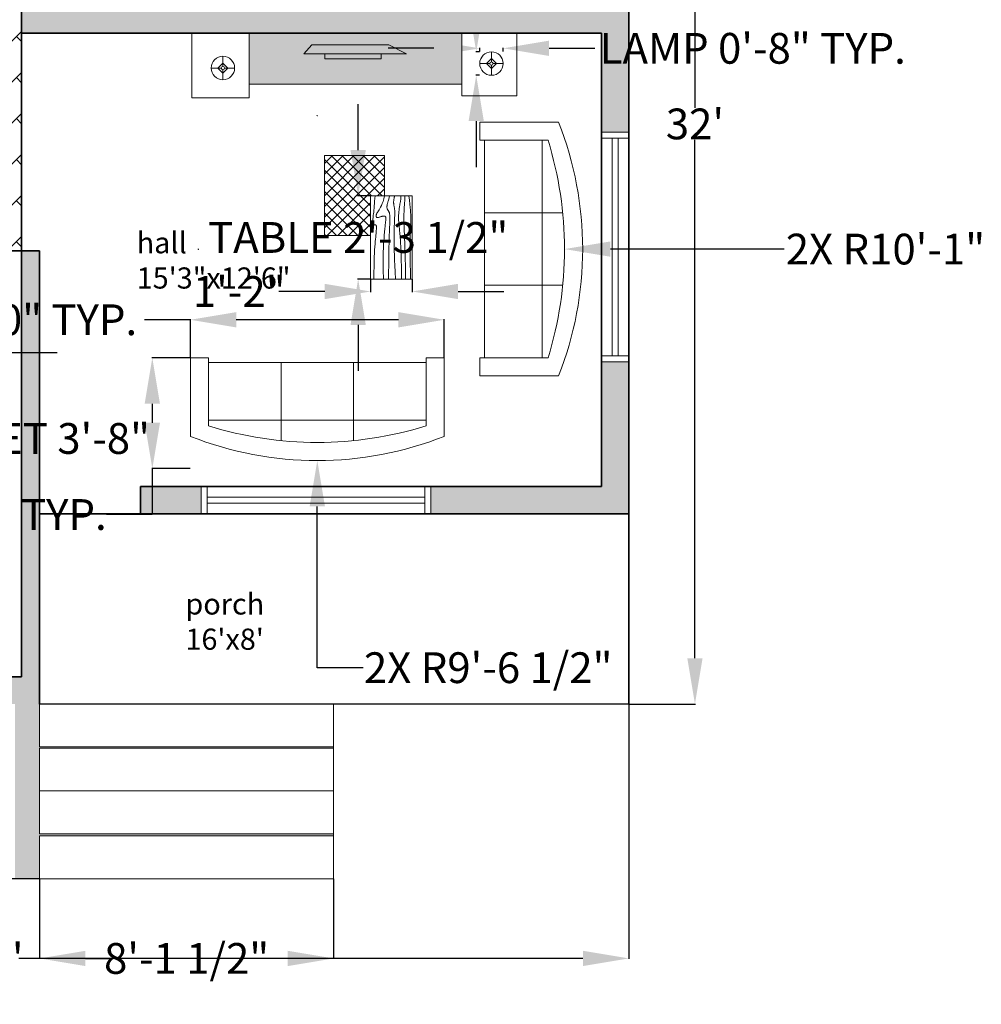
# Model space of a CAD drawing. Units: inches. Extents: x 1031 to 1706, y 87 to 654.
# Tile 3 of 4: x 1318 to 1636, y 87 to 413. Entities that reach past the tile are written whole.
import ezdxf

# ---------------------------------------------------------------- set-up
doc = ezdxf.new("R2010")
doc.units = ezdxf.units.IN
doc.header["$MEASUREMENT"] = 0
for name, color, linetype, lineweight in [('A-ANNO-DIMS', 2, 'Continuous', 18), ('A-AREA-IDEN', 7, 'Continuous', 25), ('A-EQPM', 9, 'Continuous', 18), ('A-EQPM-PATT', 18, 'Continuous', 13), ('A-FLOR', 7, 'Continuous', 25), ('A-FLOR-PATT', 152, 'Continuous', 13), ('A-FLOR-STRS', 7, 'Continuous', 18), ('A-FURN', 215, 'Continuous', 18), ('A-FURN-PATT', 41, 'Continuous', 13), ('A-GLAZ', 4, 'Continuous', 18), ('A-WALL', 7, 'Continuous', 35), ('A-WALL-PATT', 18, 'Continuous', 13)]:
    doc.layers.add(name, color=color, linetype=linetype, lineweight=lineweight)
doc.styles.get("Standard").update_dxf_attribs({"font": 'arial.ttf'})
doc.dimstyles.get("Standard").update_dxf_attribs({"dimtxt": 10.18, "dimasz": 15.18, "dimexe": 0.18, "dimexo": 0.0625, "dimgap": 0.09, "dimtad": 0, "dimtih": 1, "dimtoh": 1, "dimdec": 0, "dimzin": 0, "dimdsep": 46, "dimlunit": 3, "dimtxsty": 'Standard', "dimcen": 0.09, "dimadec": 0, "dimazin": 0, "dimtfac": 1, "dimtdec": 0, "dimtofl": 0, "dimtmove": 0, "dimatfit": 3, "dimfxl": 1, "dimtolj": 1, "dimtzin": 0, "dimarcsym": 0})

# ---------------------------------------------------------------- blocks, each defined once
blk = doc.blocks.new('Sofa - Roundback 7 ft.')
for p, q in [((-12.00002, -32.4421), (-12.00003, -6.5971)), ((11.99997, -32.4421), (11.99998, -6.5971)), ((-36.000027, -34), (-36.000027, -11.4696)), ((35.99998, -34), (35.99998, -11.4696)), ((-35.999844, -13.3819), (35.9998, -13.3819)), ((-36.000027, -32.4421), (35.99998, -32.4421))]:
    blk.add_line(p, q)
for points in [[(-36.000027, -34), (-42.000027, -34), (-42.000027, -8)], [(41.99998, -8), (41.99998, -34), (35.99998, -34)]]:
    blk.add_lwpolyline(points)
for centre, radius, start, end in [((0, -114.25), 114.25, 68.43141, 111.5686), ((-0.00001, -127.1968), 121.1968, 72.72033, 107.2797)]:
    blk.add_arc(centre, radius, start, end)
blk = doc.blocks.new('Table - Rectangular Woodgrain 60 x 30 in.')
for p, q in [((0, 0), (0, -30)), ((60, 0), (0, 0)), ((60, -30), (60, 0)), ((0, -30), (60, -30))]:
    blk.add_line(p, q)
for points in [[(0, -2.4), (4.8155, -2.418), (9.0302, -2.4688), (12.709, -2.5477), (15.9167, -2.65), (18.7181, -2.7711), (21.1781, -2.9063), (23.3616, -3.0508), (25.3333, -3.2), (27.1477, -3.3495), (28.8172, -3.4958), (30.3437, -3.636), (31.7291, -3.7667), (32.9756, -3.8849), (34.0849, -3.9875), (35.059, -4.0714), (35.9, -4.1334), (36.6114, -4.1711), (37.2041, -4.1854), (37.6906, -4.1779), (38.0833, -4.15), (38.3948, -4.1034), (38.6375, -4.0396), (38.8239, -3.9602), (38.9666, -3.8667), (39.0764, -3.7608), (39.1573, -3.6448), (39.2116, -3.521), (39.2416, -3.3917), (39.2498, -3.2593), (39.2385, -3.1261), (39.21, -2.9944), (39.1666, -2.8667), (39.111, -2.7447), (39.0468, -2.6281), (38.978, -2.5163), (38.9083, -2.4083), (38.8418, -2.3035), (38.7823, -2.201), (38.7337, -2.1001), (38.7, -2), (38.6844, -1.9003), (38.6875, -1.8021), (38.7094, -1.707), (38.75, -1.6167), (38.8094, -1.5326), (38.8875, -1.4563), (38.9844, -1.3893), (39.1, -1.3333), (39.2351, -1.2896), (39.3937, -1.2583), (39.5804, -1.2396), (39.8, -1.2333), (40.057, -1.2396), (40.3562, -1.2583), (40.7023, -1.2896), (41.1, -1.3333), (41.5547, -1.3895), (42.0755, -1.4573), (42.6721, -1.5361), (43.3542, -1.625), (44.1316, -1.7233), (45.014, -1.8302), (46.0114, -1.9449), (47.1333, -2.0667), (48.3862, -2.1947), (49.7625, -2.3281), (51.2513, -2.4663), (52.8416, -2.6083), (54.5226, -2.7535), (56.2833, -2.9011), (58.1127, -3.0501), (60, -3.2)], [(0, -9.2), (6.5759, -9.0858), (11.9385, -9.0365), (16.2527, -9.0418), (19.6833, -9.0917), (22.3952, -9.1759), (24.5531, -9.2844), (26.322, -9.4069), (27.8666, -9.5333), (29.3241, -9.6553), (30.7203, -9.7719), (32.0532, -9.8837), (33.3208, -9.9917), (34.5213, -10.0965), (35.6526, -10.199), (36.7128, -10.2999), (37.7, -10.4), (38.6129, -10.4996), (39.4531, -10.5969), (40.223, -10.6895), (40.925, -10.775), (41.5613, -10.8512), (42.1344, -10.9156), (42.6465, -10.966), (43.1, -11), (43.4976, -11.0158), (43.8437, -11.0136), (44.143, -10.9942), (44.4, -10.9583), (44.6195, -10.9069), (44.8062, -10.8406), (44.9648, -10.7603), (45.1, -10.6667), (45.2155, -10.5598), (45.3114, -10.4365), (45.3871, -10.2929), (45.4416, -10.125), (45.4743, -9.929), (45.4844, -9.7011), (45.4709, -9.4371), (45.4333, -9.1333), (45.3716, -8.7883), (45.2896, -8.4104), (45.1919, -8.0107), (45.0833, -7.6), (44.9685, -7.1893), (44.8521, -6.7896), (44.7388, -6.4117), (44.6333, -6.0667), (44.54, -5.7628), (44.4614, -5.4979), (44.4001, -5.2675), (44.3583, -5.0667), (44.3384, -4.8909), (44.3427, -4.7354), (44.3736, -4.5956), (44.4333, -4.4667), (44.5236, -4.3453), (44.6427, -4.2333), (44.7884, -4.1339), (44.9583, -4.05), (45.1501, -3.9849), (45.3614, -3.9417), (45.59, -3.9234), (45.8333, -3.9333), (46.0915, -3.9749), (46.3734, -4.0531), (46.6906, -4.1736), (47.0542, -4.3417), (47.4756, -4.5629), (47.9661, -4.8427), (48.5372, -5.1866), (49.2, -5.6), (49.9676, -6.0844), (50.8594, -6.625), (51.8965, -7.2031), (53.1, -7.8), (54.491, -8.3969), (56.0906, -8.975), (57.9199, -9.5156), (60, -10)], [(0, -12.8), (5.1847, -12.9322), (9.6213, -13.0323), (13.3963, -13.1059), (16.5958, -13.1583), (19.3063, -13.1952), (21.614, -13.2219), (23.6054, -13.2439), (25.3666, -13.2667), (26.9728, -13.2947), (28.4531, -13.3281), (29.8256, -13.3663), (31.1083, -13.4083), (32.3191, -13.4535), (33.476, -13.501), (34.597, -13.5501), (35.7, -13.6), (36.7984, -13.6497), (37.8875, -13.6979), (38.9578, -13.743), (40, -13.7833), (41.0047, -13.8174), (41.9625, -13.8438), (42.864, -13.8607), (43.7, -13.8667), (44.4631, -13.8604), (45.1552, -13.8417), (45.7801, -13.8104), (46.3416, -13.7667), (46.8439, -13.7104), (47.2906, -13.6417), (47.6858, -13.5604), (48.0333, -13.4667), (48.3375, -13.3608), (48.6042, -13.2448), (48.8396, -13.121), (49.05, -12.9917), (49.2417, -12.8593), (49.4208, -12.7261), (49.5937, -12.5944), (49.7667, -12.4667), (49.9452, -12.3451), (50.1323, -12.2313), (50.3303, -12.1268), (50.5416, -12.0333), (50.7686, -11.9524), (51.0135, -11.8854), (51.2788, -11.8341), (51.5666, -11.8), (51.8785, -11.7843), (52.2116, -11.7865), (52.562, -11.8059), (52.926, -11.8417), (53.2998, -11.8931), (53.6795, -11.9594), (54.0614, -12.0397), (54.4416, -12.1333), (54.8223, -12.2401), (55.2293, -12.3625), (55.6942, -12.5037), (56.2489, -12.6667), (56.9251, -12.8547), (57.7545, -13.0708), (58.7689, -13.3182), (60, -13.6)], [(0, -18), (5.124, -17.7273), (9.6609, -17.5057), (13.6705, -17.3303), (17.2125, -17.1958), (20.3467, -17.0973), (23.1328, -17.0297), (25.6307, -16.9878), (27.9, -16.9667), (29.9928, -16.9617), (31.9302, -16.9703), (33.7254, -16.9907), (35.3917, -17.0208), (36.9423, -17.0588), (38.3906, -17.1026), (39.7499, -17.1503), (41.0333, -17.2), (42.2519, -17.2496), (43.4073, -17.2969), (44.4986, -17.3395), (45.525, -17.375), (46.4858, -17.4012), (47.3802, -17.4156), (48.2074, -17.416), (48.9667, -17.4), (49.6583, -17.3662), (50.2872, -17.3167), (50.8595, -17.2547), (51.3812, -17.1833), (51.8584, -17.1057), (52.2971, -17.025), (52.7034, -16.9443), (53.0833, -16.8667), (53.443, -16.7951), (53.789, -16.7313), (54.128, -16.6768), (54.4666, -16.6334), (54.8115, -16.6024), (55.1693, -16.5854), (55.5465, -16.5841), (55.95, -16.6), (56.3828, -16.6337), (56.8346, -16.6823), (57.2915, -16.7418), (57.7396, -16.8084), (58.165, -16.878), (58.5539, -16.9469), (58.8924, -17.0111), (59.1666, -17.0667), (59.3679, -17.1107), (59.5078, -17.1438), (59.6032, -17.1675), (59.6708, -17.1833), (59.7275, -17.193), (59.7901, -17.1979), (59.8753, -17.1998), (60, -17.2)], [(0, -22.4), (8.0098, -22.2501), (14.4094, -22.1011), (19.4168, -21.9535), (23.25, -21.8083), (26.1269, -21.6663), (28.2656, -21.5281), (29.884, -21.3947), (31.2, -21.2667), (32.3967, -21.1448), (33.5172, -21.0292), (34.5697, -20.9198), (35.5625, -20.8167), (36.5037, -20.7198), (37.4015, -20.6292), (38.2642, -20.5448), (39.1, -20.4667), (39.9164, -20.3951), (40.7187, -20.3313), (41.5117, -20.2768), (42.3, -20.2333), (43.0883, -20.2024), (43.8812, -20.1854), (44.6836, -20.1841), (45.5, -20.2), (46.3328, -20.234), (47.1747, -20.2844), (48.0163, -20.3488), (48.8479, -20.425), (49.66, -20.5106), (50.4429, -20.6031), (51.1872, -20.7004), (51.8833, -20.8), (52.5246, -20.8999), (53.1166, -20.9995), (53.6681, -21.0983), (54.1875, -21.1958), (54.6834, -21.2919), (55.1646, -21.3859), (55.6394, -21.4777), (56.1167, -21.5667), (56.6028, -21.6515), (57.0961, -21.7266), (57.5929, -21.7852), (58.0896, -21.8208), (58.5823, -21.8268), (59.0674, -21.7964), (59.5412, -21.723), (60, -21.6)], [(0, -25.2), (8.6355, -25.0504), (15.7026, -24.9031), (21.4049, -24.7606), (25.9458, -24.625), (29.529, -24.4988), (32.3578, -24.3844), (34.6359, -24.284), (36.5667, -24.2), (38.3213, -24.1341), (39.9417, -24.0854), (41.437, -24.0523), (42.8167, -24.0333), (44.0901, -24.0268), (45.2667, -24.0313), (46.3557, -24.0451), (47.3667, -24.0667), (48.309, -24.0947), (49.1928, -24.1287), (50.0284, -24.168), (50.826, -24.2125), (51.5959, -24.2617), (52.3483, -24.3151), (53.0935, -24.3725), (53.8417, -24.4334), (54.6009, -24.497), (55.3699, -24.561), (56.1454, -24.6226), (56.9239, -24.6792), (57.7021, -24.7279), (58.4764, -24.7662), (59.2435, -24.7911), (60, -24.8)], [(0, -28.8), (5.6867, -28.6681), (10.45, -28.5698), (14.407, -28.5012), (17.675, -28.4584), (20.3711, -28.4374), (22.6125, -28.4344), (24.5164, -28.4455), (26.2, -28.4667), (27.762, -28.4947), (29.2276, -28.5281), (30.6033, -28.5663), (31.8958, -28.6084), (33.1118, -28.6535), (34.2578, -28.7011), (35.3405, -28.7501), (36.3666, -28.8), (37.3443, -28.8497), (38.288, -28.8974), (39.2137, -28.9412), (40.1375, -28.9792), (41.0753, -29.0093), (42.0432, -29.0297), (43.0572, -29.0384), (44.1333, -29.0333), (45.2936, -29.0114), (46.5843, -28.9641), (48.0579, -28.8816), (49.7666, -28.7542), (51.7629, -28.5721), (54.0989, -28.3255), (56.8272, -28.0048), (60, -27.6)]]:
    blk.add_lwpolyline(points)
blk = doc.blocks.new('*D14')
at = {"layer": 'A-ANNO-DIMS', "color": 0, "lineweight": -2, "transparency": 16777216}
for p, q in [((1519.66, 570.4), (1541.66, 570.4)), ((1541.48, 555.22), (1541.48, 383.69)), ((1541.48, 201.58), (1541.48, 373.11)), ((1519.66, 186.4), (1541.66, 186.4))]:
    blk.add_line(p, q, dxfattribs=at)
at = {"layer": 'A-ANNO-DIMS', "color": 0, "transparency": 16777216}
for points in [[(1538.95, 555.22), (1544.01, 555.22), (1541.48, 570.4)], [(1538.95, 201.58), (1544.01, 201.58), (1541.48, 186.4)]]:
    blk.add_solid(points, dxfattribs=at)
at = {"layer": 'Defpoints', "color": 0, "transparency": 16777216}
for p in [(1519.6, 570.4), (1519.6, 186.4), (1541.48, 186.4)]:
    blk.add_point(p, dxfattribs=at)
at = {"layer": 'A-ANNO-DIMS', "color": 0, "transparency": 16777216, "insert": (1541.48, 378.4), "char_height": 10.18, "attachment_point": 5}
blk.add_mtext("\\A1;32'", dxfattribs=at)
blk = doc.blocks.new('Lamp - Table')
for p, q in [((0, 7), (0, 1)), ((-1, 0), (-7, 0)), ((0, 3), (-3, 0)), ((-3, 0), (0, -3)), ((3, 0), (0, 3)), ((0, -3), (3, 0)), ((1, 0), (7, 0)), ((0, -1), (0, -7))]:
    blk.add_line(p, q)
for radius in [7, 1]:
    blk.add_circle((0, 0), radius)
blk = doc.blocks.new('WIN-72IN')
for p, q in [((0, 0), (0, 9)), ((2, 0), (2, 9)), ((74, 0), (74, 9)), ((76, 0), (76, 9)), ((2, 5.5), (74, 5.5)), ((2, 3.5), (74, 3.5))]:
    blk.add_line(p, q)
blk = doc.blocks.new('*D26')
at = {"layer": 'A-ANNO-DIMS', "color": 0, "lineweight": -2, "transparency": 16777216}
for p, q in [((1455.08, 403.42), (1439.9, 403.42)), ((1470.26, 402.32), (1470.26, 403.6)), ((1478.02, 402.32), (1478.02, 403.6)), ((1493.2, 403.42), (1508.38, 403.42))]:
    blk.add_line(p, q, dxfattribs=at)
at = {"layer": 'A-ANNO-DIMS', "color": 0, "transparency": 16777216}
for points in [[(1455.08, 405.95), (1455.08, 400.89), (1470.26, 403.42)], [(1493.2, 405.95), (1493.2, 400.89), (1478.02, 403.42)]]:
    blk.add_solid(points, dxfattribs=at)
at = {"layer": 'Defpoints', "color": 0, "transparency": 16777216}
for p in [(1470.26, 402.26), (1478.02, 403.42), (1478.02, 402.26)]:
    blk.add_point(p, dxfattribs=at)
at = {"layer": 'A-ANNO-DIMS', "color": 0, "transparency": 16777216, "insert": (1560.61, 403.42), "char_height": 10.18, "attachment_point": 5}
blk.add_mtext('\\A1;LAMP 0\'-8" TYP.', dxfattribs=at)
blk = doc.blocks.new('*D27')
at = {"layer": 'A-ANNO-DIMS', "color": 0, "lineweight": -2, "transparency": 16777216}
for p, q in [((1469.1, 417.44), (1469.1, 432.62)), ((1469.1, 432.62), (1484.28, 432.62)), ((1470.2, 402.26), (1468.92, 402.26)), ((1470.2, 394.5), (1468.92, 394.5)), ((1469.1, 379.32), (1469.1, 364.14))]:
    blk.add_line(p, q, dxfattribs=at)
at = {"layer": 'A-ANNO-DIMS', "color": 0, "transparency": 16777216}
for points in [[(1466.57, 417.44), (1471.63, 417.44), (1469.1, 402.26)], [(1466.57, 379.32), (1471.63, 379.32), (1469.1, 394.5)]]:
    blk.add_solid(points, dxfattribs=at)
at = {"layer": 'Defpoints', "color": 0, "transparency": 16777216}
for p in [(1469.1, 402.26), (1470.26, 402.26), (1470.26, 394.5)]:
    blk.add_point(p, dxfattribs=at)
at = {"layer": 'A-ANNO-DIMS', "color": 0, "transparency": 16777216, "insert": (1515.39, 432.62), "char_height": 10.18, "attachment_point": 5}
blk.add_mtext('\\A1;0\'-8" TYP.', dxfattribs=at)
blk = doc.blocks.new('*D28')
at = {"layer": 'A-ANNO-DIMS', "color": 0, "lineweight": -2, "transparency": 16777216}
for p, q in [((1374.5, 313.58), (1359.32, 313.58)), ((1374.5, 301.04), (1374.5, 313.76)), ((1443.32, 313.58), (1389.68, 313.58)), ((1458.5, 301.04), (1458.5, 313.76))]:
    blk.add_line(p, q, dxfattribs=at)
at = {"layer": 'A-ANNO-DIMS', "color": 0, "transparency": 16777216}
for points in [[(1389.68, 316.11), (1389.68, 311.05), (1374.5, 313.58)], [(1443.32, 316.11), (1443.32, 311.05), (1458.5, 313.58)]]:
    blk.add_solid(points, dxfattribs=at)
at = {"layer": 'Defpoints', "color": 0, "transparency": 16777216}
for p in [(1374.5, 313.58), (1374.5, 300.98), (1458.5, 300.98)]:
    blk.add_point(p, dxfattribs=at)
at = {"layer": 'A-ANNO-DIMS', "color": 0, "transparency": 16777216, "insert": (1306.9, 313.58), "char_height": 10.18, "attachment_point": 5}
blk.add_mtext('\\A1;SOFA 7\'-0" TYP.', dxfattribs=at)
blk = doc.blocks.new('*D29')
at = {"layer": 'A-ANNO-DIMS', "color": 0, "lineweight": -2, "transparency": 16777216}
for p, q in [((1374.44, 300.98), (1361.72, 300.98)), ((1361.9, 285.8), (1361.9, 279.49)), ((1374.44, 264.31), (1361.72, 264.31)), ((1361.9, 264.31), (1361.9, 249.13)), ((1361.9, 249.13), (1346.72, 249.13))]:
    blk.add_line(p, q, dxfattribs=at)
at = {"layer": 'A-ANNO-DIMS', "color": 0, "transparency": 16777216}
for points in [[(1359.37, 285.8), (1364.43, 285.8), (1361.9, 300.98)], [(1359.37, 279.49), (1364.43, 279.49), (1361.9, 264.31)]]:
    blk.add_solid(points, dxfattribs=at)
at = {"layer": 'Defpoints', "color": 0, "transparency": 16777216}
for p in [(1374.5, 300.98), (1361.9, 264.31), (1374.5, 264.31)]:
    blk.add_point(p, dxfattribs=at)
at = {"layer": 'A-ANNO-DIMS', "color": 0, "transparency": 16777216, "insert": (1303.75, 249.13), "char_height": 10.18, "attachment_point": 5}
blk.add_mtext('\\A1;3\'-0 1/2" TYP.', dxfattribs=at)
blk = doc.blocks.new('*D30')
at = {"layer": 'A-ANNO-DIMS', "color": 0, "lineweight": -2, "transparency": 16777216}
for p, q in [((1300.12, 296.19), (1306.8, 296.19)), ((1306.62, 281.01), (1306.62, 279.65)), ((1306.62, 267.58), (1306.62, 268.93)), ((1300.12, 252.4), (1306.8, 252.4))]:
    blk.add_line(p, q, dxfattribs=at)
at = {"layer": 'A-ANNO-DIMS', "color": 0, "transparency": 16777216}
for points in [[(1304.09, 281.01), (1309.15, 281.01), (1306.62, 296.19)], [(1304.09, 267.58), (1309.15, 267.58), (1306.62, 252.4)]]:
    blk.add_solid(points, dxfattribs=at)
at = {"layer": 'Defpoints', "color": 0, "transparency": 16777216}
for p in [(1300.06, 296.19), (1306.62, 296.19), (1300.06, 252.4)]:
    blk.add_point(p, dxfattribs=at)
at = {"layer": 'A-ANNO-DIMS', "color": 0, "transparency": 16777216, "insert": (1306.62, 274.29), "char_height": 10.18, "attachment_point": 5}
blk.add_mtext('\\A1;DINING SET 3\'-8"', dxfattribs=at)
blk = doc.blocks.new('*D31')
at = {"layer": 'A-ANNO-DIMS', "color": 0, "lineweight": -2, "transparency": 16777216}
for p, q in [((1258.41, 302.75), (1243.23, 302.75)), ((1273.59, 296.25), (1273.59, 302.93)), ((1300.06, 296.25), (1300.06, 302.93)), ((1315.24, 302.75), (1330.42, 302.75))]:
    blk.add_line(p, q, dxfattribs=at)
at = {"layer": 'A-ANNO-DIMS', "color": 0, "transparency": 16777216}
for points in [[(1258.41, 305.28), (1258.41, 300.22), (1273.59, 302.75)], [(1315.24, 305.28), (1315.24, 300.22), (1300.06, 302.75)]]:
    blk.add_solid(points, dxfattribs=at)
at = {"layer": 'Defpoints', "color": 0, "transparency": 16777216}
for p in [(1273.59, 302.75), (1273.59, 296.19), (1300.06, 296.19)]:
    blk.add_point(p, dxfattribs=at)
at = {"layer": 'A-ANNO-DIMS', "color": 0, "transparency": 16777216, "insert": (1217.66, 302.75), "char_height": 10.18, "attachment_point": 5}
blk.add_mtext('\\A1;2\'-2 1/2"', dxfattribs=at)
blk = doc.blocks.new('*D38')
at = {"layer": 'A-ANNO-DIMS', "color": 0, "lineweight": -2, "transparency": 16777216}
for p, q in [((1430.03, 369.75), (1430.03, 384.93)), ((1434.09, 354.57), (1429.85, 354.57)), ((1434.09, 327.06), (1429.85, 327.06)), ((1430.03, 311.88), (1430.03, 296.7))]:
    blk.add_line(p, q, dxfattribs=at)
at = {"layer": 'A-ANNO-DIMS', "color": 0, "transparency": 16777216}
for points in [[(1427.5, 369.75), (1432.56, 369.75), (1430.03, 354.57)], [(1427.5, 311.88), (1432.56, 311.88), (1430.03, 327.06)]]:
    blk.add_solid(points, dxfattribs=at)
at = {"layer": 'Defpoints', "color": 0, "transparency": 16777216}
for p in [(1430.03, 354.57), (1434.15, 354.57), (1434.15, 327.06)]:
    blk.add_point(p, dxfattribs=at)
at = {"layer": 'A-ANNO-DIMS', "color": 0, "transparency": 16777216, "insert": (1430.03, 340.82), "char_height": 10.18, "attachment_point": 5}
blk.add_mtext('\\A1;TABLE 2\'-3 1/2"', dxfattribs=at)
blk = doc.blocks.new('*D39')
at = {"layer": 'A-ANNO-DIMS', "color": 0, "lineweight": -2, "transparency": 16777216}
for p, q in [((1434.15, 327), (1434.15, 322.76)), ((1447.91, 327), (1447.91, 322.76)), ((1418.97, 322.94), (1403.79, 322.94)), ((1463.09, 322.94), (1478.27, 322.94))]:
    blk.add_line(p, q, dxfattribs=at)
at = {"layer": 'A-ANNO-DIMS', "color": 0, "transparency": 16777216}
for points in [[(1418.97, 325.47), (1418.97, 320.41), (1434.15, 322.94)], [(1463.09, 325.47), (1463.09, 320.41), (1447.91, 322.94)]]:
    blk.add_solid(points, dxfattribs=at)
at = {"layer": 'Defpoints', "color": 0, "transparency": 16777216}
for p in [(1434.15, 327.06), (1447.91, 327.06), (1434.15, 322.94)]:
    blk.add_point(p, dxfattribs=at)
at = {"layer": 'A-ANNO-DIMS', "color": 0, "transparency": 16777216, "insert": (1390.65, 322.94), "char_height": 10.18, "attachment_point": 5}
blk.add_mtext('\\A1;1\'-2"', dxfattribs=at)
blk = doc.blocks.new('*D40')
at = {"layer": 'A-ANNO-DIMS', "color": 0, "lineweight": -2, "transparency": 16777216}
for p, q in [((1080.61, 327.33), (1080.61, 102.02)), ((1519.6, 186.33), (1519.6, 102.02)), ((1095.79, 102.2), (1282.53, 102.2)), ((1504.42, 102.2), (1317.68, 102.2))]:
    blk.add_line(p, q, dxfattribs=at)
at = {"layer": 'A-ANNO-DIMS', "color": 0, "transparency": 16777216}
for points in [[(1095.79, 104.73), (1095.79, 99.67), (1080.61, 102.2)], [(1504.42, 104.73), (1504.42, 99.67), (1519.6, 102.2)]]:
    blk.add_solid(points, dxfattribs=at)
at = {"layer": 'Defpoints', "color": 0, "transparency": 16777216}
for p in [(1080.61, 327.4), (1519.6, 186.4), (1519.6, 102.2)]:
    blk.add_point(p, dxfattribs=at)
at = {"layer": 'A-ANNO-DIMS', "color": 0, "transparency": 16777216, "insert": (1300.1, 102.2), "char_height": 10.18, "attachment_point": 5}
blk.add_mtext('\\A1;36\'-7"', dxfattribs=at)
blk = doc.blocks.new('*D41')
at = {"layer": 'A-ANNO-DIMS', "color": 0, "lineweight": -2, "transparency": 16777216}
for p, q in [((1129.54, 570.4), (1054.03, 570.4)), ((1054.21, 555.22), (1054.21, 354.79)), ((1054.21, 143.78), (1054.21, 344.21)), ((1324.54, 128.6), (1054.03, 128.6))]:
    blk.add_line(p, q, dxfattribs=at)
at = {"layer": 'A-ANNO-DIMS', "color": 0, "transparency": 16777216}
for points in [[(1051.68, 555.22), (1056.74, 555.22), (1054.21, 570.4)], [(1051.68, 143.78), (1056.74, 143.78), (1054.21, 128.6)]]:
    blk.add_solid(points, dxfattribs=at)
at = {"layer": 'Defpoints', "color": 0, "transparency": 16777216}
for p in [(1054.21, 570.4), (1129.6, 570.4), (1324.6, 128.6)]:
    blk.add_point(p, dxfattribs=at)
at = {"layer": 'A-ANNO-DIMS', "color": 0, "transparency": 16777216, "insert": (1054.21, 349.5), "char_height": 10.18, "attachment_point": 5}
blk.add_mtext('\\A1;36\'-10"', dxfattribs=at)
blk = doc.blocks.new('*D43')
at = {"layer": 'A-ANNO-DIMS', "color": 0, "lineweight": -2, "transparency": 16777216}
for p, q in [((1324.6, 128.54), (1324.6, 102.02)), ((1421.89, 128.54), (1421.89, 102.02)), ((1339.78, 102.2), (1347.76, 102.2)), ((1406.71, 102.2), (1398.73, 102.2))]:
    blk.add_line(p, q, dxfattribs=at)
at = {"layer": 'A-ANNO-DIMS', "color": 0, "transparency": 16777216}
for points in [[(1339.78, 104.73), (1339.78, 99.67), (1324.6, 102.2)], [(1406.71, 104.73), (1406.71, 99.67), (1421.89, 102.2)]]:
    blk.add_solid(points, dxfattribs=at)
at = {"layer": 'Defpoints', "color": 0, "transparency": 16777216}
for p in [(1324.6, 128.6), (1421.89, 128.6), (1421.89, 102.2)]:
    blk.add_point(p, dxfattribs=at)
at = {"layer": 'A-ANNO-DIMS', "color": 0, "transparency": 16777216, "insert": (1373.25, 102.2), "char_height": 10.18, "attachment_point": 5}
blk.add_mtext('\\A1;8\'-1 1/2"', dxfattribs=at)
blk = doc.blocks.new('*D46')
at = {"layer": 'A-ANNO-DIMS', "color": 0, "lineweight": -2, "transparency": 16777216}
for p, q in [((1377.05, 336.98), (1377.23, 336.98)), ((1377.14, 336.89), (1377.14, 337.07)), ((1571.05, 336.98), (1513.51, 336.98))]:
    blk.add_line(p, q, dxfattribs=at)
at = {"layer": 'A-ANNO-DIMS', "color": 0, "transparency": 16777216}
blk.add_solid([(1513.51, 339.51), (1513.51, 334.45), (1498.33, 336.98)], dxfattribs=at)
at = {"layer": 'Defpoints', "color": 0, "transparency": 16777216}
for p in [(1377.14, 336.98), (1498.33, 336.98)]:
    blk.add_point(p, dxfattribs=at)
at = {"layer": 'A-ANNO-DIMS', "color": 0, "transparency": 16777216, "insert": (1604.52, 336.98), "char_height": 10.18, "attachment_point": 5}
blk.add_mtext('\\A1;2X R10\'-1"', dxfattribs=at)
blk = doc.blocks.new('*D47')
at = {"layer": 'A-ANNO-DIMS', "color": 0, "lineweight": -2, "transparency": 16777216}
for p, q in [((1416.5, 381.14), (1416.5, 381.32)), ((1416.41, 381.23), (1416.59, 381.23)), ((1416.5, 198.43), (1416.5, 251.8)), ((1431.68, 198.43), (1416.5, 198.43))]:
    blk.add_line(p, q, dxfattribs=at)
at = {"layer": 'A-ANNO-DIMS', "color": 0, "transparency": 16777216}
blk.add_solid([(1419.03, 251.8), (1413.97, 251.8), (1416.5, 266.98)], dxfattribs=at)
at = {"layer": 'Defpoints', "color": 0, "transparency": 16777216}
for p in [(1416.5, 381.23), (1416.5, 266.98)]:
    blk.add_point(p, dxfattribs=at)
at = {"layer": 'A-ANNO-DIMS', "color": 0, "transparency": 16777216, "insert": (1473.06, 198.43), "char_height": 10.18, "attachment_point": 5}
blk.add_mtext('\\A1;2X R9\'-6 1/2"', dxfattribs=at)

msp = doc.modelspace()

# ---------------------------------------------------------------- hatches: boundary and pattern name
at = {"layer": 'A-EQPM-PATT'}
h = msp.add_hatch(color=256, dxfattribs=at)
h.dxf.hatch_style = 1
h.paths.add_polyline_path([(1440.18, 404.55), (1414.65, 404.55), (1412.04, 401.55), (1445.97, 401.55)])
h = msp.add_hatch(color=256, dxfattribs=at)
h.dxf.hatch_style = 1
h.paths.add_polyline_path([(1437.65, 401.55), (1418.94, 401.55), (1418.94, 399.97), (1437.65, 399.97)])
at = {"layer": 'A-FLOR-PATT'}
h = msp.add_hatch(dxfattribs=at)
h.set_pattern_fill('AR-HBONE', color=256, scale=2.4)
h.paths.add_polyline_path([(1372.6, 507.4), (1330.6, 507.4), (1330.6, 471.4), (1276.6, 471.4), (1276.6, 408.4), (1276.6, 336.4), (1318.6, 336.4), (1318.6, 417.4), (1372.6, 417.4)])
h = msp.add_hatch(dxfattribs=at)
h.set_pattern_fill('AR-HBONE', color=256, scale=860)
h.paths.add_polyline_path([(1438.74, 367.92), (1418.85, 367.92), (1418.85, 341.42), (1434.15, 341.42), (1434.15, 354.57), (1438.74, 354.57)])
h = msp.add_hatch(dxfattribs=at)
h.set_pattern_fill('ANSI37', color=256, scale=20)
h.paths.add_polyline_path([(1434.15, 354.57), (1438.74, 354.57), (1438.74, 367.92), (1418.85, 367.92), (1418.85, 341.42), (1434.15, 341.42)])
at = {"layer": 'A-FURN-PATT'}
h = msp.add_hatch(color=256, dxfattribs=at)
h.dxf.hatch_style = 1
h.paths.add_polyline_path([(1464.32, 408.4), (1393.94, 408.4), (1393.94, 391.57), (1464.32, 391.57)])
at = {"layer": 'A-WALL-PATT'}
h = msp.add_hatch(color=256, dxfattribs=at)
h.dxf.hatch_style = 1
h.paths.add_polyline_path([(1324.6, 336.4), (1318.6, 336.4), (1318.6, 327.4), (1318.6, 195.4), (1256.53, 195.4), (1256.53, 186.4), (1316.43, 186.4), (1316.43, 128.6), (1324.6, 128.6), (1324.6, 142.78), (1421.89, 142.78), (1421.89, 143.49), (1324.6, 143.49), (1324.6, 157.67), (1324.6, 171.8), (1421.89, 171.8), (1421.89, 172.21), (1324.6, 172.21), (1324.6, 186.4)])
h.paths.add_polyline_path([(1378.07, 258.4), (1358.04, 258.4), (1358.04, 249.4), (1378.07, 249.4)], flags=17)
h.paths.add_polyline_path([(1519.6, 299.69), (1510.6, 299.69), (1510.6, 258.4), (1454.07, 258.4), (1454.07, 249.4), (1519.6, 249.4)])
h.paths.add_polyline_path([(1519.6, 456.87), (1510.6, 456.87), (1510.6, 417.4), (1372.6, 417.4), (1318.6, 417.4), (1318.6, 408.4), (1510.6, 408.4), (1510.6, 375.69), (1519.6, 375.69)])
h.paths.add_polyline_path([(1276.6, 372.4), (1270.65, 372.4), (1270.65, 336.4), (1138.6, 336.4), (1092.08, 336.4), (1092.08, 346.4), (1080.61, 346.4), (1080.61, 327.4), (1129.6, 327.4), (1129.6, 290.93), (1138.6, 290.93), (1138.6, 291.84), (1138.6, 327.4), (1244.94, 327.4), (1276.6, 327.4)])
h.paths.add_polyline_path([(1276.6, 417.4), (1138.6, 417.4), (1138.6, 438.03), (1129.6, 438.03), (1129.6, 417.4), (1080.61, 417.4), (1080.61, 398.4), (1092.08, 398.4), (1092.08, 408.4), (1138.6, 408.4), (1276.6, 408.4)])
h.paths.add_polyline_path([(1180.53, 195.4), (1138.6, 195.4), (1138.6, 214.93), (1129.6, 214.93), (1129.6, 186.4), (1180.53, 186.4)])
h.paths.add_polyline_path([(1519.6, 570.4), (1489.02, 570.4), (1489.02, 561.4), (1510.6, 561.4), (1510.6, 532.87), (1519.6, 532.87)])
h.paths.add_polyline_path([(1413.02, 570.4), (1365.47, 570.4), (1365.47, 561.4), (1372.6, 561.4), (1372.6, 507.4), (1372.6, 417.4), (1378.6, 417.4), (1378.6, 561.4), (1413.02, 561.4)])
h.paths.add_polyline_path([(1289.42, 570.4), (1242.6, 570.4), (1242.6, 561.4), (1270.6, 561.4), (1270.6, 471.4), (1291.02, 471.4), (1291.02, 477.4), (1276.6, 477.4), (1276.6, 561.4), (1289.42, 561.4)])
h.paths.add_polyline_path([(1337.47, 570.4), (1317.42, 570.4), (1317.42, 561.4), (1324.6, 561.4), (1324.6, 471.4), (1330.6, 471.4), (1330.6, 507.4), (1338.54, 507.4), (1338.54, 513.4), (1330.6, 513.4), (1330.6, 561.4), (1337.47, 561.4)])
h.paths.add_polyline_path([(1138.6, 561.4), (1166.6, 561.4), (1166.6, 570.4), (1129.6, 570.4), (1129.6, 514.03), (1138.6, 514.03)])

# ---------------------------------------------------------------- linework, layer by layer
at = {"layer": 'A-EQPM'}
for p, q in [((1414.65, 404.55), (1412.04, 401.55)), ((1440.18, 404.55), (1414.65, 404.55)), ((1445.97, 401.55), (1440.18, 404.55)), ((1412.04, 401.55), (1445.97, 401.55))]:
    msp.add_line(p, q, dxfattribs=at)
msp.add_lwpolyline([(1418.94, 401.55), (1437.65, 401.55), (1437.65, 399.97), (1418.94, 399.97)], close=True, dxfattribs=at)
at = {"layer": 'A-FLOR'}
msp.add_line((1519.6, 186.4), (1324.6, 186.4), dxfattribs=at)
at = {"layer": 'A-FLOR-STRS'}
for p, q in [((1421.89, 186.4), (1421.89, 128.6)), ((1316.43, 128.6), (1324.6, 128.6))]:
    msp.add_line(p, q, dxfattribs=at)
for points in [[(1421.89, 172.21), (1324.6, 172.21), (1324.6, 186.4), (1519.18, 186.4)], [(1421.89, 157.62), (1324.6, 157.62), (1324.6, 171.8), (1421.89, 171.8)], [(1421.89, 143.49), (1324.6, 143.49), (1324.6, 157.67), (1421.89, 157.67)], [(1421.89, 128.6), (1324.6, 128.6), (1324.6, 142.78), (1421.89, 142.78)]]:
    msp.add_lwpolyline(points, dxfattribs=at)
at = {"layer": 'A-FURN'}
for p, q in [((1389.82, 408.4), (1464.32, 408.4)), ((1393.94, 391.57), (1393.94, 408.4)), ((1464.32, 408.4), (1464.32, 391.57)), ((1464.32, 391.57), (1393.94, 391.57)), ((1438.74, 367.92), (1418.85, 367.92)), ((1418.85, 367.92), (1418.85, 341.42)), ((1438.74, 354.57), (1438.74, 367.92)), ((1418.85, 341.42), (1434.15, 341.42))]:
    msp.add_line(p, q, dxfattribs=at)
for points in [[(1393.94, 408.4), (1374.95, 408.4), (1374.95, 387.07), (1393.94, 387.07)], [(1464.32, 408.4), (1482.55, 408.4), (1482.55, 387.7), (1464.32, 387.7)]]:
    msp.add_lwpolyline(points, close=True, dxfattribs=at)
at = {"layer": 'A-WALL'}
for p, q in [((1519.6, 570.4), (1519.6, 186.4)), ((1318.6, 327.4), (1318.6, 417.4)), ((1318.6, 408.4), (1510.6, 408.4)), ((1510.6, 408.4), (1510.6, 258.4)), ((1324.6, 336.4), (1276.6, 336.4)), ((1324.6, 186.4), (1324.6, 336.4)), ((1318.6, 195.4), (1318.6, 327.4)), ((1358.04, 258.4), (1510.6, 258.4)), ((1358.04, 258.4), (1358.04, 249.4)), ((1324.6, 249.4), (1519.6, 249.4)), ((1318.6, 195.4), (1138.6, 195.4))]:
    msp.add_line(p, q, dxfattribs=at)

# ---------------------------------------------------------------- block references
at = {"layer": 'A-FURN', "xscale": 0.5540798285396209, "yscale": 0.5540798285396209, "zscale": 0.5540798285396209}
for p in [(1474.14, 398.38), (1385.27, 396.9)]:
    msp.add_blockref('Lamp - Table', p, dxfattribs=at)
at = {"layer": 'A-FURN'}
for p, rotation in [((1504.33, 336.98), 270), ((1416.5, 266.98), 180)]:
    msp.add_blockref('Sofa - Roundback 7 ft.', p, dxfattribs=dict(at, rotation=rotation))
at = {"layer": 'A-FURN', "xscale": 0.4585028725585568, "yscale": 0.4585028725585568, "zscale": 0.4585028725585568, "rotation": 90}
msp.add_blockref('Table - Rectangular Woodgrain 60 x 30 in.', (1434.15, 327.06), dxfattribs=at)
at = {"layer": 'A-GLAZ'}
for p, rotation in [((1519.6, 299.69), 90.00000000000088), ((1454.07, 258.4), 180)]:
    msp.add_blockref('WIN-72IN', p, dxfattribs=dict(at, rotation=rotation))

# ---------------------------------------------------------------- texts
at = {"layer": 'A-AREA-IDEN', "char_height": 7, "attachment_point": 1}
for s, insert in [('hall\\P15\'3"x12\'6"', (1356.72, 342.57)), ("porch\\P16'x8'", (1372.85, 223.03))]:
    msp.add_mtext_dynamic_manual_height_columns(s, width=113.8004, gutter_width=1, heights=[0], dxfattribs=dict(at, insert=insert))

# ---------------------------------------------------------------- dimensions: what is measured, and where the dimension line sits
at = {"layer": 'A-ANNO-DIMS'}
for base, p1, p2, angle, override, picture, middle in [((1054.21, 570.4), (1324.6, 128.6), (1129.6, 570.4), 90, {"dimdec": 1, "dimlfac": 1, "dimrnd": 0, "dimzin": 1, "dimdsep": 46, "dimlunit": 4, "dimfrac": 2}, '*D41', (1054.21, 349.5)), ((1541.48, 186.4), (1519.6, 570.4), (1519.6, 186.4), 90, {"dimclrd": 0, "dimclre": 0, "dimclrt": 0}, '*D14', (1541.48, 378.4)), ((1434.15, 322.94), (1447.91, 327.06), (1434.15, 327.06), 180, {"dimdec": 1, "dimlfac": 1, "dimrnd": 0, "dimzin": 1, "dimdsep": 46, "dimlunit": 4, "dimfrac": 2}, '*D39', (1390.65, 322.94)), ((1273.59, 302.75), (1300.06, 296.19), (1273.59, 296.19), 180, {"dimdec": 1, "dimlfac": 1, "dimrnd": 0, "dimzin": 1, "dimdsep": 46, "dimlunit": 4, "dimfrac": 2}, '*D31', (1217.66, 302.75))]:
    dim = msp.add_linear_dim(base=base, p1=p1, p2=p2, angle=angle, dimstyle='Standard', override=override, dxfattribs=at)
    dim.commit()
    dim.dimension.update_dxf_attribs({"geometry": picture, "text_midpoint": middle})
for base, p1, p2, angle, text, picture, middle in [((1469.1, 402.26), (1470.26, 394.5), (1470.26, 402.26), 90, '<> TYP.', '*D27', (1515.39, 432.62)), ((1430.03, 354.57), (1434.15, 327.06), (1434.15, 354.57), 90, 'TABLE <>', '*D38', (1430.03, 340.82)), ((1374.5, 313.58), (1458.5, 300.98), (1374.5, 300.98), 180, 'SOFA <> TYP.', '*D28', (1306.9, 313.58)), ((1361.9, 264.31), (1374.5, 300.98), (1374.5, 264.31), 270, '<> TYP.', '*D29', (1303.75, 249.13)), ((1306.62, 296.19), (1300.06, 252.4), (1300.06, 296.19), 90, 'DINING SET <>', '*D30', (1306.62, 274.29))]:
    dim = msp.add_linear_dim(base=base, p1=p1, p2=p2, angle=angle, text=text, dimstyle='Standard', override={"dimdec": 1, "dimlfac": 1, "dimrnd": 0, "dimzin": 1, "dimdsep": 46, "dimlunit": 4, "dimfrac": 2}, dxfattribs=at)
    dim.commit()
    dim.dimension.update_dxf_attribs({"geometry": picture, "text_midpoint": middle})
dim = msp.add_linear_dim(base=(1478.02, 403.42), p1=(1470.26, 402.26), p2=(1478.02, 402.26), text='LAMP <> TYP.', dimstyle='Standard', override={"dimdec": 1, "dimlfac": 1, "dimrnd": 0, "dimzin": 1, "dimdsep": 46, "dimlunit": 4, "dimfrac": 2}, dxfattribs=at)
dim.commit()
dim.dimension.update_dxf_attribs({"geometry": '*D26', "text_midpoint": (1560.61, 403.42)})
for center, mpoint, picture, middle in [((1416.502789, 381.22609), (1416.503, 266.97609), '*D47', (1473.05906794, 198.42609)), ((1377.14, 336.98), (1498.33, 336.98), '*D46', (1571.05, 336.98))]:
    dim = msp.add_radius_dim(center=center, mpoint=mpoint, text='2X <>', dimstyle='Standard', override={"dimdec": 1, "dimlfac": 1, "dimrnd": 0, "dimzin": 1, "dimdsep": 46, "dimlunit": 4, "dimfrac": 2}, dxfattribs=at)
    dim.commit()
    dim.dimension.update_dxf_attribs({"geometry": picture, "text_midpoint": middle, "dimtype": 164})
for base, p1, p2, picture, middle in [((1519.6, 102.2), (1080.61, 327.4), (1519.6, 186.4), '*D40', (1300.1, 102.2)), ((1421.89, 102.2), (1324.6, 128.6), (1421.89, 128.6), '*D43', (1373.25, 102.2))]:
    dim = msp.add_linear_dim(base=base, p1=p1, p2=p2, dimstyle='Standard', override={"dimdec": 1, "dimlfac": 1, "dimrnd": 0, "dimzin": 1, "dimdsep": 46, "dimlunit": 4, "dimfrac": 2}, dxfattribs=at)
    dim.commit()
    dim.dimension.update_dxf_attribs({"geometry": picture, "text_midpoint": middle})

doc.saveas('drawing.dxf')
